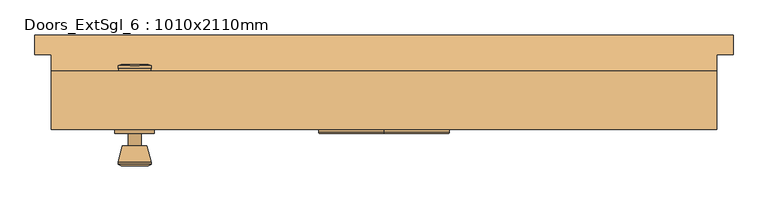
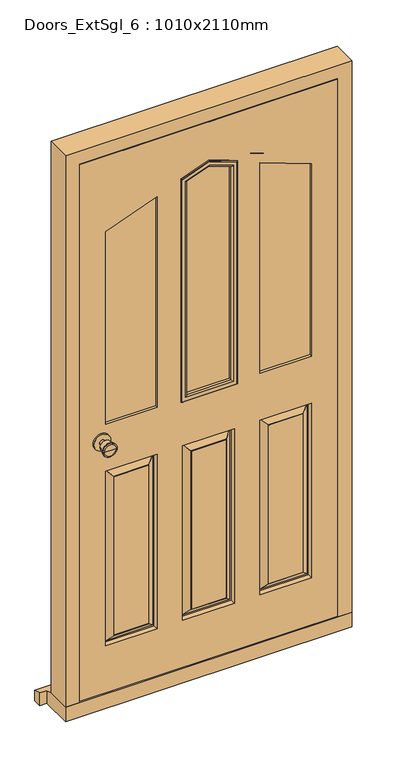
"""IFC4 building model written with IfcOpenShell, lengths in millimetres: door geometry, Doors_ExtSgl_6 : 1010x2110mm."""

from ifc_helpers import new_model, si_unit, point, frame, frame_2d, origin, place, context, project, spatial, polyline, circle_curve, ellipse_curve, trimmed, segment, composite_curve, outline, extrude, faceted_brep, source, transform, mapped, element, save
from ifc_brep_helpers import plane_surface, cylinder_surface, revolved_surface, advanced_brep


def doors_extsgl_6_1010x2110mm_b93c615f(model_context):
    return source(origin(), model_context, "Body", "SolidModel", [
        advanced_brep(
        [(-378.4666667, -18.4, 1000.0), (-368.4666667, -18.4, 1000.0), (-388.4666667, -18.4, 1000.0), (-357.9907991, -67.4, 1000.0), (-378.4666667, -67.4, 1000.0), (-398.9425342, -67.4, 1000.0), (-353.4666667, -65.5721319, 1000.0), (-403.4666667, -65.5721319, 1000.0), (-353.4666667, -62.1084537, 1000.0), (-403.4666667, -62.1084537, 1000.0), (-359.8304306, -37.4, 1000.0), (-397.1029027, -37.4, 1000.0), (-368.4666667, -37.4, 1000.0), (-388.4666667, -37.4, 1000.0)],
        [
            (0, 1),
            (1, 2, circle_curve(frame((-378.4666667, -18.4, 1000.0), z_axis=(0.0, 1.0, 0.0), x_axis=(-1.0, 0.0, 0.0)), 10.0)),
            (2, 0),
            (2, 1, circle_curve(frame((-378.4666667, -18.4, 1000.0), z_axis=(0.0, 1.0, 0.0), x_axis=(-1.0, 0.0, 0.0)), 10.0)),
            (3, 4),
            (4, 5),
            (5, 3, circle_curve(frame((-378.4666667, -67.4, 1000.0), z_axis=(0.0, -1.0, 0.0), x_axis=(-1.0, 0.0, 0.0)), 20.4758676)),
            (3, 5, circle_curve(frame((-378.4666667, -67.4, 1000.0), z_axis=(0.0, -1.0, 0.0), x_axis=(-1.0, 0.0, 0.0)), 20.4758676)),
            (6, 3),
            (5, 7),
            (7, 6, circle_curve(frame((-378.4666667, -65.5721319, 1000.0), z_axis=(0.0, -1.0, 0.0), x_axis=(-1.0, 0.0, 0.0)), 25.0)),
            (6, 7, circle_curve(frame((-378.4666667, -65.5721319, 1000.0), z_axis=(0.0, -1.0, 0.0), x_axis=(-1.0, 0.0, 0.0)), 25.0)),
            (8, 6),
            (7, 9),
            (9, 8, circle_curve(frame((-378.4666667, -62.1084537, 1000.0), z_axis=(0.0, -1.0, 0.0), x_axis=(-1.0, 0.0, 0.0)), 25.0)),
            (8, 9, circle_curve(frame((-378.4666667, -62.1084537, 1000.0), z_axis=(0.0, -1.0, 0.0), x_axis=(-1.0, 0.0, 0.0)), 25.0)),
            (10, 8),
            (9, 11),
            (11, 10, circle_curve(frame((-378.4666667, -37.4, 1000.0), z_axis=(0.0, -1.0, 0.0), x_axis=(-1.0, 0.0, 0.0)), 18.636236)),
            (10, 11, circle_curve(frame((-378.4666667, -37.4, 1000.0), z_axis=(0.0, -1.0, 0.0), x_axis=(-1.0, 0.0, 0.0)), 18.636236)),
            (12, 10),
            (11, 13),
            (13, 12, circle_curve(frame((-378.4666667, -37.4, 1000.0), z_axis=(0.0, -1.0, 0.0), x_axis=(-1.0, 0.0, 0.0)), 10.0)),
            (12, 13, circle_curve(frame((-378.4666667, -37.4, 1000.0), z_axis=(0.0, -1.0, 0.0), x_axis=(-1.0, 0.0, 0.0)), 10.0)),
            (1, 12),
            (13, 2),
        ],
        [
            plane_surface(frame((-378.4666667, -18.4, 1000.0), z_axis=(0.0, 1.0, 0.0), x_axis=(-1.0, 0.0, 0.0))),
            plane_surface(frame((-378.4666667, -67.4, 1000.0), z_axis=(0.0, -1.0, 0.0), x_axis=(-1.0, 0.0, 0.0))),
            revolved_surface(polyline([(-398.9425342, -67.4, 1000.0), (-403.4666667, -65.5721319, 1000.0)]), (-378.4666667, -18.4, 1000.0), (0.0, 1.0, 0.0)),
            cylinder_surface(frame((-378.4666667, -18.4, 1000.0), z_axis=(0.0, 1.0, 0.0), x_axis=(-1.0, 0.0, 0.0)), 25.0),
            revolved_surface(polyline([(-403.4666667, -62.1084537, 1000.0), (-397.1029027, -37.4, 1000.0)]), (-378.4666667, -18.4, 1000.0), (0.0, 1.0, 0.0)),
            plane_surface(frame((-378.4666667, -37.4, 1000.0), z_axis=(0.0, 1.0, 0.0), x_axis=(-1.0, 0.0, 0.0))),
            cylinder_surface(frame((-378.4666667, -18.4, 1000.0), z_axis=(0.0, 1.0, 0.0), x_axis=(-1.0, 0.0, 0.0)), 10.0),
        ],
        [
            (0, [[1, 2, 3]]),
            (0, [[-3, 4, -1]]),
            (1, [[5, 6, 7]]),
            (1, [[-6, -5, 8]]),
            (2, [[9, -7, 10, 11]]),
            (2, [[-10, -8, -9, 12]]),
            (3, [[13, -11, 14, 15]]),
            (3, [[-14, -12, -13, 16]]),
            (4, [[17, -15, 18, 19]]),
            (4, [[-18, -16, -17, 20]]),
            (5, [[21, -19, 22, 23]]),
            (5, [[-22, -20, -21, 24]]),
            (6, [[25, -23, 26, -2]]),
            (6, [[-26, -24, -25, -4]]),
        ],
    ),
        extrude(outline(composite_curve([segment(trimmed(circle_curve(frame_2d((1000.0, -378.4666667)), 30.0), [point((1000.0, -408.4666667))], [point((1000.0, -348.4666667))], False, "CARTESIAN"), True, "CONTINUOUS"), segment(trimmed(circle_curve(frame_2d((1000.0, -378.4666667)), 30.0), [point((1000.0, -348.4666667))], [point((1000.0, -408.4666667))], False, "CARTESIAN"), True, "CONTINUOUS")], self_intersect=False)), frame((0.0, -18.4, 0.0), z_axis=(0.0, 1.0, 0.0), x_axis=(0.0, 0.0, 1.0)), (0.0, 0.0, 1.0), 6.0),
        advanced_brep(
        [(-378.4666667, 37.6, 1000.0), (-388.4666667, 37.6, 1000.0), (-368.4666667, 37.6, 1000.0), (-357.9907991, 86.6, 1000.0), (-398.9425342, 86.6, 1000.0), (-378.4666667, 86.6, 1000.0), (-353.4666667, 84.7721319, 1000.0), (-403.4666667, 84.7721319, 1000.0), (-353.4666667, 81.3084537, 1000.0), (-403.4666667, 81.3084537, 1000.0), (-359.8304306, 56.6, 1000.0), (-397.1029027, 56.6, 1000.0), (-368.4666667, 56.6, 1000.0), (-388.4666667, 56.6, 1000.0)],
        [
            (0, 1),
            (1, 2, circle_curve(frame((-378.4666667, 37.6, 1000.0), z_axis=(0.0, -1.0, 0.0), x_axis=(-1.0, 0.0, 0.0)), 10.0)),
            (2, 0),
            (2, 1, circle_curve(frame((-378.4666667, 37.6, 1000.0), z_axis=(0.0, -1.0, 0.0), x_axis=(-1.0, 0.0, 0.0)), 10.0)),
            (3, 4, circle_curve(frame((-378.4666667, 86.6, 1000.0), z_axis=(0.0, 1.0, 0.0), x_axis=(-1.0, 0.0, 0.0)), 20.4758676)),
            (4, 5),
            (5, 3),
            (4, 3, circle_curve(frame((-378.4666667, 86.6, 1000.0), z_axis=(0.0, 1.0, 0.0), x_axis=(-1.0, 0.0, 0.0)), 20.4758676)),
            (6, 7, circle_curve(frame((-378.4666667, 84.7721319, 1000.0), z_axis=(0.0, 1.0, 0.0), x_axis=(-1.0, 0.0, 0.0)), 25.0)),
            (7, 4),
            (3, 6),
            (7, 6, circle_curve(frame((-378.4666667, 84.7721319, 1000.0), z_axis=(0.0, 1.0, 0.0), x_axis=(-1.0, 0.0, 0.0)), 25.0)),
            (8, 9, circle_curve(frame((-378.4666667, 81.3084537, 1000.0), z_axis=(0.0, 1.0, 0.0), x_axis=(-1.0, 0.0, 0.0)), 25.0)),
            (9, 7),
            (6, 8),
            (9, 8, circle_curve(frame((-378.4666667, 81.3084537, 1000.0), z_axis=(0.0, 1.0, 0.0), x_axis=(-1.0, 0.0, 0.0)), 25.0)),
            (10, 11, circle_curve(frame((-378.4666667, 56.6, 1000.0), z_axis=(0.0, 1.0, 0.0), x_axis=(-1.0, 0.0, 0.0)), 18.636236)),
            (11, 9),
            (8, 10),
            (11, 10, circle_curve(frame((-378.4666667, 56.6, 1000.0), z_axis=(0.0, 1.0, 0.0), x_axis=(-1.0, 0.0, 0.0)), 18.636236)),
            (12, 13, circle_curve(frame((-378.4666667, 56.6, 1000.0), z_axis=(0.0, 1.0, 0.0), x_axis=(-1.0, 0.0, 0.0)), 10.0)),
            (13, 11),
            (10, 12),
            (13, 12, circle_curve(frame((-378.4666667, 56.6, 1000.0), z_axis=(0.0, 1.0, 0.0), x_axis=(-1.0, 0.0, 0.0)), 10.0)),
            (1, 13),
            (12, 2),
        ],
        [
            plane_surface(frame((-378.4666667, 37.6, 1000.0), z_axis=(0.0, -1.0, 0.0), x_axis=(-1.0, 0.0, 0.0))),
            plane_surface(frame((-378.4666667, 86.6, 1000.0), z_axis=(0.0, 1.0, 0.0), x_axis=(-1.0, 0.0, 0.0))),
            revolved_surface(polyline([(-398.9425342, 86.6, 1000.0), (-403.4666667, 84.7721319, 1000.0)]), (-378.4666667, 37.6, 1000.0), (0.0, -1.0, 0.0)),
            cylinder_surface(frame((-378.4666667, 37.6, 1000.0), z_axis=(0.0, -1.0, 0.0), x_axis=(-1.0, 0.0, 0.0)), 25.0),
            revolved_surface(polyline([(-403.4666667, 81.3084537, 1000.0), (-397.1029027, 56.6, 1000.0)]), (-378.4666667, 37.6, 1000.0), (0.0, -1.0, 0.0)),
            plane_surface(frame((-378.4666667, 56.6, 1000.0), z_axis=(0.0, -1.0, 0.0), x_axis=(-1.0, 0.0, 0.0))),
            cylinder_surface(frame((-378.4666667, 37.6, 1000.0), z_axis=(0.0, -1.0, 0.0), x_axis=(-1.0, 0.0, 0.0)), 10.0),
        ],
        [
            (0, [[1, 2, 3]]),
            (0, [[-3, 4, -1]]),
            (1, [[5, 6, 7]]),
            (1, [[8, -7, -6]]),
            (2, [[9, 10, -5, 11]]),
            (2, [[12, -11, -8, -10]]),
            (3, [[13, 14, -9, 15]]),
            (3, [[16, -15, -12, -14]]),
            (4, [[17, 18, -13, 19]]),
            (4, [[20, -19, -16, -18]]),
            (5, [[21, 22, -17, 23]]),
            (5, [[24, -23, -20, -22]]),
            (6, [[-2, 25, -21, 26]]),
            (6, [[-4, -26, -24, -25]]),
        ],
    ),
        extrude(outline(composite_curve([segment(trimmed(circle_curve(frame_2d((1000.0, -378.4666667)), 30.0), [point((1000.0, -408.4666667))], [point((1000.0, -348.4666667))], False, "CARTESIAN"), True, "CONTINUOUS"), segment(trimmed(circle_curve(frame_2d((1000.0, -378.4666667)), 30.0), [point((1000.0, -348.4666667))], [point((1000.0, -408.4666667))], False, "CARTESIAN"), True, "CONTINUOUS")], self_intersect=False)), frame((0.0, 31.6, 0.0), z_axis=(0.0, 1.0, 0.0), x_axis=(0.0, 0.0, 1.0)), (0.0, 0.0, 1.0), 6.0),
        faceted_brep([(434.5333333, 76.6, 54.5), (505.0333333, 76.6, 54.5), (505.0333333, -12.4, 54.5), (456.5333333, -12.4, 54.5), (456.5333333, 34.6, 54.5), (434.5333333, 34.6, 54.5), (434.5333333, 76.6, 2039.5), (-434.4666667, 76.6, 2039.5), (-434.4666667, 76.6, 54.5), (-504.9666667, 76.6, 54.5), (-504.9666667, 76.6, 2110.0), (505.0333333, 76.6, 2110.0), (505.0333333, -12.4, 2110.0), (-504.9666667, -12.4, 2110.0), (-504.9666667, -12.4, 54.5), (-456.4666667, -12.4, 54.5), (-456.4666667, -12.4, 2061.5), (456.5333333, -12.4, 2061.5), (456.5333333, 34.6, 2061.5), (-456.4666667, 34.6, 2061.5), (-456.4666667, 34.6, 54.5), (-434.4666667, 34.6, 54.5), (-434.4666667, 34.6, 2039.5), (434.5333333, 34.6, 2039.5)], [[[0, 1, 2, 3, 4, 5]], [[1, 0, 6, 7, 8, 9, 10, 11]], [[2, 1, 11, 12]], [[3, 2, 12, 13, 14, 15, 16, 17]], [[4, 3, 17, 18]], [[5, 4, 18, 19, 20, 21, 22, 23]], [[0, 5, 23, 6]], [[8, 7, 22, 21]], [[9, 8, 21, 20, 15, 14]], [[10, 9, 14, 13]], [[16, 15, 20, 19]], [[11, 10, 13, 12]], [[17, 16, 19, 18]], [[7, 6, 23, 22]]]),
        faceted_brep([(453.5333333, -12.4, 58.5), (453.5333333, -12.4, 2058.5), (-454.3916961, -12.4, 2058.5), (-454.3916961, -12.4, 58.5), (-91.1333333, -12.4, 1058.5), (-91.1333333, -12.4, 1875.318047), (0.0333333, -12.4, 1908.5), (91.2, -12.4, 1875.318047), (91.2, -12.4, 1058.5), (363.5333333, -12.4, 1058.5), (181.2, -12.4, 1058.5), (181.2, -12.4, 1842.5607259), (363.5333333, -12.4, 1776.1968198), (-181.1333333, -12.4, 1842.5607259), (-181.1333333, -12.4, 1058.5), (-363.4666667, -12.4, 1058.5), (-363.4666667, -12.4, 1776.1968198), (-181.1333333, -12.4, 883.5), (-181.1333333, -12.4, 233.5), (-363.4666667, -12.4, 233.5), (-363.4666667, -12.4, 883.5), (363.5333333, -12.4, 883.5), (363.5333333, -12.4, 233.5), (181.2, -12.4, 233.5), (181.2, -12.4, 883.5), (91.2, -12.4, 883.5), (91.2, -12.4, 233.5), (-91.1333333, -12.4, 233.5), (-91.1333333, -12.4, 883.5), (-211.1333333, -12.4, 263.5), (-211.1333333, -12.4, 853.5), (-333.4666667, -12.4, 853.5), (-333.4666667, -12.4, 263.5), (333.5333333, -12.4, 263.5), (333.5333333, -12.4, 853.5), (211.2, -12.4, 853.5), (211.2, -12.4, 263.5), (61.2, -12.4, 263.5), (61.2, -12.4, 853.5), (-61.1333333, -12.4, 853.5), (-61.1333333, -12.4, 263.5), (453.5333333, 31.6, 58.5), (-454.3916961, 31.6, 58.5), (-454.3916961, 31.6, 2058.5), (453.5333333, 31.6, 2058.5), (-91.1333333, 31.6, 1058.5), (91.2, 31.6, 1058.5), (91.2, 31.6, 1875.318047), (0.0333333, 31.6, 1908.5), (-91.1333333, 31.6, 1875.318047), (363.5333333, 31.6, 1058.5), (363.5333333, 31.6, 1776.1968198), (181.2, 31.6, 1842.5607259), (181.2, 31.6, 1058.5), (-181.1333333, 31.6, 1842.5607259), (-363.4666667, 31.6, 1776.1968198), (-363.4666667, 31.6, 1058.5), (-181.1333333, 31.6, 1058.5), (181.2, 31.6, 883.5), (181.2, 31.6, 233.5), (363.5333333, 31.6, 233.5), (363.5333333, 31.6, 883.5), (-363.4666667, 31.6, 883.5), (-363.4666667, 31.6, 233.5), (-181.1333333, 31.6, 233.5), (-181.1333333, 31.6, 883.5), (-91.1333333, 31.6, 883.5), (-91.1333333, 31.6, 233.5), (91.2, 31.6, 233.5), (91.2, 31.6, 883.5), (211.2, 31.6, 263.5), (211.2, 31.6, 853.5), (333.5333333, 31.6, 853.5), (333.5333333, 31.6, 263.5), (-333.4666667, 31.6, 263.5), (-333.4666667, 31.6, 853.5), (-211.1333333, 31.6, 853.5), (-211.1333333, 31.6, 263.5), (-61.1333333, 31.6, 263.5), (-61.1333333, 31.6, 853.5), (61.2, 31.6, 853.5), (61.2, 31.6, 263.5), (184.2, 16.6, 880.5), (184.2, 16.6, 236.5), (209.2, 30.6, 855.5), (209.2, 30.6, 261.5), (189.2, 16.6, 241.5), (189.2, 16.6, 875.5), (211.2, 30.6, 263.5), (211.2, 30.6, 853.5), (360.5333333, 16.6, 236.5), (335.5333333, 30.6, 261.5), (355.5333333, 16.6, 241.5), (333.5333333, 30.6, 263.5), (360.5333333, 16.6, 880.5), (335.5333333, 30.6, 855.5), (355.5333333, 16.6, 875.5), (333.5333333, 30.6, 853.5), (-360.4666667, 16.6, 880.5), (-360.4666667, 16.6, 236.5), (-335.4666667, 30.6, 855.5), (-335.4666667, 30.6, 261.5), (-355.4666667, 16.6, 241.5), (-355.4666667, 16.6, 875.5), (-333.4666667, 30.6, 263.5), (-333.4666667, 30.6, 853.5), (-184.1333333, 16.6, 236.5), (-209.1333333, 30.6, 261.5), (-189.1333333, 16.6, 241.5), (-211.1333333, 30.6, 263.5), (-184.1333333, 16.6, 880.5), (-209.1333333, 30.6, 855.5), (-189.1333333, 16.6, 875.5), (-211.1333333, 30.6, 853.5), (-211.1333333, -11.4, 263.5), (-211.1333333, -11.4, 853.5), (-189.1333333, 2.6, 241.5), (-189.1333333, 2.6, 875.5), (-209.1333333, -11.4, 855.5), (-209.1333333, -11.4, 261.5), (-184.1333333, 2.6, 880.5), (-184.1333333, 2.6, 236.5), (-333.4666667, -11.4, 853.5), (-355.4666667, 2.6, 875.5), (-335.4666667, -11.4, 855.5), (-360.4666667, 2.6, 880.5), (-333.4666667, -11.4, 263.5), (-355.4666667, 2.6, 241.5), (-335.4666667, -11.4, 261.5), (-360.4666667, 2.6, 236.5), (360.5333333, 2.6, 880.5), (360.5333333, 2.6, 236.5), (335.5333333, -11.4, 855.5), (335.5333333, -11.4, 261.5), (355.5333333, 2.6, 241.5), (355.5333333, 2.6, 875.5), (333.5333333, -11.4, 263.5), (333.5333333, -11.4, 853.5), (184.2, 2.6, 236.5), (209.2, -11.4, 261.5), (189.2, 2.6, 241.5), (211.2, -11.4, 263.5), (184.2, 2.6, 880.5), (209.2, -11.4, 855.5), (189.2, 2.6, 875.5), (211.2, -11.4, 853.5), (-61.1333333, 30.6, 263.5), (-61.1333333, 30.6, 853.5), (-83.1333333, 16.6, 241.5), (-83.1333333, 16.6, 875.5), (-63.1333333, 30.6, 855.5), (-63.1333333, 30.6, 261.5), (-88.1333333, 16.6, 880.5), (-88.1333333, 16.6, 236.5), (61.2, 30.6, 853.5), (83.2, 16.6, 875.5), (63.2, 30.6, 855.5), (88.2, 16.6, 880.5), (61.2, 30.6, 263.5), (83.2, 16.6, 241.5), (63.2, 30.6, 261.5), (88.2, 16.6, 236.5), (88.2, 2.6, 880.5), (88.2, 2.6, 236.5), (63.2, -11.4, 855.5), (63.2, -11.4, 261.5), (83.2, 2.6, 241.5), (83.2, 2.6, 875.5), (61.2, -11.4, 263.5), (61.2, -11.4, 853.5), (-88.1333333, 2.6, 236.5), (-63.1333333, -11.4, 261.5), (-83.1333333, 2.6, 241.5), (-61.1333333, -11.4, 263.5), (-88.1333333, 2.6, 880.5), (-63.1333333, -11.4, 855.5), (-83.1333333, 2.6, 875.5), (-61.1333333, -11.4, 853.5)], [[[0, 1, 2, 3], [4, 5, 6, 7, 8], [9, 10, 11, 12], [13, 14, 15, 16], [17, 18, 19, 20], [21, 22, 23, 24], [25, 26, 27, 28]], [[29, 30, 31, 32]], [[33, 34, 35, 36]], [[37, 38, 39, 40]], [[41, 42, 43, 44], [45, 46, 47, 48, 49], [50, 51, 52, 53], [54, 55, 56, 57], [58, 59, 60, 61], [62, 63, 64, 65], [66, 67, 68, 69]], [[70, 71, 72, 73]], [[74, 75, 76, 77]], [[78, 79, 80, 81]], [[1, 0, 41, 44]], [[2, 1, 44, 43]], [[3, 2, 43, 42]], [[0, 3, 42, 41]], [[5, 4, 45, 49]], [[6, 5, 49, 48]], [[7, 6, 48, 47]], [[8, 7, 47, 46]], [[4, 8, 46, 45]], [[10, 9, 50, 53]], [[11, 10, 53, 52]], [[12, 11, 52, 51]], [[9, 12, 51, 50]], [[14, 13, 54, 57]], [[15, 14, 57, 56]], [[16, 15, 56, 55]], [[13, 16, 55, 54]], [[82, 83, 59, 58]], [[84, 85, 86, 87]], [[70, 88, 89, 71]], [[59, 83, 90, 60]], [[86, 85, 91, 92]], [[88, 70, 73, 93]], [[60, 90, 94, 61]], [[92, 91, 95, 96]], [[93, 73, 72, 97]], [[82, 58, 61, 94]], [[83, 82, 94, 90], [87, 86, 92, 96]], [[84, 87, 96, 95]], [[85, 84, 95, 91], [89, 88, 93, 97]], [[71, 89, 97, 72]], [[98, 99, 63, 62]], [[100, 101, 102, 103]], [[74, 104, 105, 75]], [[63, 99, 106, 64]], [[102, 101, 107, 108]], [[104, 74, 77, 109]], [[64, 106, 110, 65]], [[108, 107, 111, 112]], [[109, 77, 76, 113]], [[98, 62, 65, 110]], [[99, 98, 110, 106], [103, 102, 108, 112]], [[100, 103, 112, 111]], [[101, 100, 111, 107], [105, 104, 109, 113]], [[75, 105, 113, 76]], [[114, 115, 30, 29]], [[116, 117, 118, 119]], [[17, 120, 121, 18]], [[30, 115, 122, 31]], [[118, 117, 123, 124]], [[120, 17, 20, 125]], [[31, 122, 126, 32]], [[124, 123, 127, 128]], [[125, 20, 19, 129]], [[114, 29, 32, 126]], [[119, 118, 124, 128], [115, 114, 126, 122]], [[116, 119, 128, 127]], [[121, 120, 125, 129], [117, 116, 127, 123]], [[18, 121, 129, 19]], [[130, 131, 22, 21]], [[132, 133, 134, 135]], [[33, 136, 137, 34]], [[22, 131, 138, 23]], [[134, 133, 139, 140]], [[136, 33, 36, 141]], [[23, 138, 142, 24]], [[140, 139, 143, 144]], [[141, 36, 35, 145]], [[130, 21, 24, 142]], [[131, 130, 142, 138], [135, 134, 140, 144]], [[132, 135, 144, 143]], [[133, 132, 143, 139], [137, 136, 141, 145]], [[34, 137, 145, 35]], [[146, 147, 79, 78]], [[148, 149, 150, 151]], [[66, 152, 153, 67]], [[79, 147, 154, 80]], [[150, 149, 155, 156]], [[152, 66, 69, 157]], [[80, 154, 158, 81]], [[156, 155, 159, 160]], [[157, 69, 68, 161]], [[146, 78, 81, 158]], [[151, 150, 156, 160], [147, 146, 158, 154]], [[148, 151, 160, 159]], [[153, 152, 157, 161], [149, 148, 159, 155]], [[67, 153, 161, 68]], [[162, 163, 26, 25]], [[164, 165, 166, 167]], [[37, 168, 169, 38]], [[26, 163, 170, 27]], [[166, 165, 171, 172]], [[168, 37, 40, 173]], [[27, 170, 174, 28]], [[172, 171, 175, 176]], [[173, 40, 39, 177]], [[162, 25, 28, 174]], [[163, 162, 174, 170], [167, 166, 172, 176]], [[164, 167, 176, 175]], [[165, 164, 175, 171], [169, 168, 173, 177]], [[38, 169, 177, 39]]]),
        faceted_brep([(530.0333333, 131.6, 0.0), (530.0333333, 131.6, 38.5947221), (530.0333333, 101.6, 47.2703282), (530.0333333, 101.6, 0.0), (-529.9666667, 131.6, 38.5947221), (-529.9666667, 131.6, 0.0), (-529.9666667, 101.6, 0.0), (-529.9666667, 101.6, 47.2703282), (505.0333333, 101.6, 0.0), (505.0333333, -12.4, 0.0), (-504.9666667, -12.4, 0.0), (-504.9666667, 101.6, 0.0), (-504.9666667, 101.6, 47.2703282), (-504.9666667, 76.6, 54.5), (505.0333333, 76.6, 54.5), (505.0333333, 101.6, 47.2703282), (-504.9666667, -12.4, 54.5), (505.0333333, -12.4, 54.5)], [[[0, 1, 2, 3]], [[4, 5, 6, 7]], [[5, 0, 3, 8, 9, 10, 11, 6]], [[1, 0, 5, 4]], [[1, 4, 7, 12, 13, 14, 15, 2]], [[13, 16, 17, 14]], [[16, 10, 9, 17]], [[12, 11, 10, 16, 13]], [[11, 12, 7, 6]], [[8, 15, 14, 17, 9]], [[15, 8, 3, 2]]]),
        extrude(outline(polyline([(1058.5, -91.1333333), (1058.5, 91.2), (1875.318047, 91.2), (1908.5, 0.0333333), (1875.318047, -91.1333333), (1058.5, -91.1333333)])), frame((0.0, -2.4, 0.0), z_axis=(0.0, 1.0, 0.0), x_axis=(0.0, 0.0, 1.0)), (0.0, 0.0, 1.0), 24.0),
        extrude(outline(polyline([(1776.1968198, 363.5333333), (1842.5607259, 181.2), (1058.5, 181.2), (1058.5, 363.5333333), (1776.1968198, 363.5333333)])), frame((0.0, -2.4, 0.0), z_axis=(0.0, 1.0, 0.0), x_axis=(0.0, 0.0, 1.0)), (0.0, 0.0, 1.0), 24.0),
        extrude(outline(polyline([(1058.5, -181.1333333), (1842.5607259, -181.1333333), (1776.1968198, -363.4666667), (1058.5, -363.4666667), (1058.5, -181.1333333)])), frame((0.0, -2.4, 0.0), z_axis=(0.0, 1.0, 0.0), x_axis=(0.0, 0.0, 1.0)), (0.0, 0.0, 1.0), 24.0),
        advanced_brep(
        [(-99.1333333, 35.6, 1050.5), (-99.1333333, 31.6, 1050.5), (-99.1333333, 31.6, 1880.9197073), (-99.1333333, 35.6, 1880.9197073), (-97.1333333, 37.6, 1052.5), (-97.1333333, 37.6, 1879.5192922), (-79.1333333, 32.6, 1070.5), (-84.1333333, 37.6, 1065.5), (-84.1333333, 37.6, 1870.4165942), (-79.1333333, 32.6, 1866.9155565), (-79.1333333, 21.6, 1070.5), (-79.1333333, 21.6, 1866.9155565), (-91.1333333, 31.6, 1058.5), (-91.1333333, 21.6, 1058.5), (-91.1333333, 21.6, 1875.318047), (-91.1333333, 31.6, 1875.318047), (0.0333333, 31.6, 1917.0134222), (0.0333333, 35.6, 1917.0134222), (0.0333333, 37.6, 1914.8850666), (0.0333333, 37.6, 1901.0507556), (0.0333333, 32.6, 1895.7298667), (0.0333333, 21.6, 1895.7298667), (0.0333333, 21.6, 1908.5), (0.0333333, 31.6, 1908.5), (99.2, 31.6, 1880.9197073), (99.2, 35.6, 1880.9197073), (97.2, 37.6, 1879.5192922), (97.2, 37.6, 1052.5), (84.2, 37.6, 1870.4165942), (84.2, 37.6, 1065.5), (79.2, 32.6, 1866.9155565), (79.2, 21.6, 1866.9155565), (91.2, 21.6, 1875.318047), (91.2, 21.6, 1058.5), (79.2, 21.6, 1070.5), (91.2, 31.6, 1875.318047), (99.2, 31.6, 1050.5), (91.2, 31.6, 1058.5), (99.2, 35.6, 1050.5), (79.2, 32.6, 1070.5)],
        [
            (0, 1),
            (1, 2),
            (2, 3),
            (3, 0),
            (4, 0, ellipse_curve(frame((-97.1333333, 35.6, 1052.5), z_axis=(-0.7071067811865476, 0.0, 0.7071067811865474), x_axis=(-0.7071067811865471, 0.0, -0.7071067811865478)), 2.8284271, 2.0)),
            (3, 5, ellipse_curve(frame((-97.1333333, 35.6, 1879.5192922), z_axis=(-0.5735764363510456, 0.0, -0.8191520442889918), x_axis=(0.8191520442889916, 0.0, -0.5735764363510464)), 2.4415492, 2.0)),
            (5, 4),
            (6, 7, ellipse_curve(frame((-84.1333333, 32.6, 1065.5), z_axis=(-0.7071067811865476, 0.0, 0.7071067811865474), x_axis=(-0.7071067811865471, 0.0, -0.7071067811865478)), 7.0710678, 5.0)),
            (7, 8),
            (8, 9, ellipse_curve(frame((-84.1333333, 32.6, 1870.4165942), z_axis=(-0.5735764363510456, 0.0, -0.8191520442889918), x_axis=(0.8191520442889916, 0.0, -0.5735764363510464)), 6.1038729, 5.0)),
            (9, 6),
            (10, 6),
            (9, 11),
            (11, 10),
            (12, 13),
            (13, 14),
            (14, 15),
            (15, 12),
            (2, 16),
            (16, 17),
            (17, 3),
            (17, 18, ellipse_curve(frame((0.0333333, 35.6, 1914.8850666), z_axis=(-1.0, 0.0, 0.0), x_axis=(0.0, 0.0, -0.9999999999999999)), 2.1283555, 2.0)),
            (18, 5),
            (8, 19),
            (19, 20, ellipse_curve(frame((0.0333333, 32.6, 1901.0507556), z_axis=(-1.0, 0.0, 0.0), x_axis=(0.0, 0.0, -0.9999999999999999)), 5.3208889, 5.0)),
            (20, 9),
            (20, 21),
            (21, 11),
            (14, 22),
            (22, 23),
            (23, 15),
            (16, 24),
            (24, 25),
            (25, 17),
            (25, 26, ellipse_curve(frame((97.2, 35.6, 1879.5192922), z_axis=(-0.5735764363510465, 0.0, 0.8191520442889915), x_axis=(-0.8191520442889916, 0.0, -0.5735764363510464)), 2.4415492, 2.0)),
            (26, 18),
            (26, 27),
            (27, 4),
            (28, 19),
            (7, 29),
            (29, 28),
            (28, 30, ellipse_curve(frame((84.2, 32.6, 1870.4165942), z_axis=(-0.5735764363510465, 0.0, 0.8191520442889915), x_axis=(-0.8191520442889916, 0.0, -0.5735764363510464)), 6.1038729, 5.0)),
            (30, 20),
            (30, 31),
            (31, 21),
            (32, 22),
            (13, 33),
            (33, 32),
            (31, 34),
            (34, 10),
            (32, 35),
            (35, 23),
            (1, 36),
            (36, 24),
            (35, 37),
            (37, 12),
            (36, 38),
            (38, 25),
            (38, 27, ellipse_curve(frame((97.2, 35.6, 1052.5), z_axis=(0.7071067811865474, 0.0, 0.7071067811865476), x_axis=(-0.7071067811865475, 0.0, 0.7071067811865475)), 2.8284271, 2.0)),
            (29, 39, ellipse_curve(frame((84.2, 32.6, 1065.5), z_axis=(0.7071067811865474, 0.0, 0.7071067811865476), x_axis=(-0.7071067811865475, 0.0, 0.7071067811865475)), 7.0710678, 5.0)),
            (39, 30),
            (39, 34),
            (33, 37),
            (0, 38),
            (6, 39),
        ],
        [
            plane_surface(frame((-99.1333333, 31.6, 1050.5), z_axis=(-1.0, 0.0, 0.0), x_axis=(0.0, 0.0, 1.0))),
            cylinder_surface(frame((-97.1333333, 35.6, 1058.5), z_axis=(0.0, 0.0, -1.0), x_axis=(-1.0, 0.0, 0.0)), 2.0),
            cylinder_surface(frame((-84.1333333, 32.6, 1058.5), z_axis=(0.0, 0.0, -1.0), x_axis=(-1.0, 0.0, 0.0)), 5.0),
            plane_surface(frame((-79.1333333, 32.6, 1070.5), z_axis=(1.0, 0.0, 0.0), x_axis=(0.0, 0.0, 1.0))),
            plane_surface(frame((-91.1333333, 21.6, 1058.5), z_axis=(-1.0, 0.0, 0.0), x_axis=(0.0, 0.0, 1.0))),
            plane_surface(frame((-99.1333333, 31.6, 1880.9197073), z_axis=(-0.3420201433256681, 0.0, 0.9396926207859086), x_axis=(0.9396926207859086, 0.0, 0.3420201433256681))),
            cylinder_surface(frame((-93.1854542, 35.6, 1880.9562027), z_axis=(-0.9396926207859082, 0.0, -0.3420201433256694), x_axis=(-0.3420201433256694, 0.0, 0.9396926207859082)), 2.0),
            cylinder_surface(frame((-88.7391923, 32.6, 1868.7401986), z_axis=(-0.9396926207859082, 0.0, -0.3420201433256694), x_axis=(-0.3420201433256694, 0.0, 0.9396926207859082)), 5.0),
            plane_surface(frame((-79.1333333, 32.6, 1866.9155565), z_axis=(0.34202014332567027, 0.0, -0.939692620785908), x_axis=(0.939692620785908, 0.0, 0.34202014332567027))),
            plane_surface(frame((-91.1333333, 21.6, 1875.318047), z_axis=(-0.34202014332566794, 0.0, 0.9396926207859088), x_axis=(0.9396926207859088, 0.0, 0.34202014332566794))),
            plane_surface(frame((0.0333333, 31.6, 1917.0134222), z_axis=(0.34202014332567027, 0.0, 0.9396926207859079), x_axis=(0.9396926207859079, 0.0, -0.34202014332567027))),
            cylinder_surface(frame((2.0854542, 35.6, 1914.1381557), z_axis=(-0.9396926207859086, 0.0, 0.3420201433256681), x_axis=(0.3420201433256681, 0.0, 0.9396926207859086)), 2.0),
            plane_surface(frame((0.0333333, 37.6, 1914.8850666), z_axis=(0.0, 1.0, 0.0), x_axis=(0.9396926207859083, 0.0, -0.3420201433256691))),
            cylinder_surface(frame((-2.3608077, 32.6, 1901.9221517), z_axis=(-0.9396926207859086, 0.0, 0.3420201433256681), x_axis=(0.3420201433256681, 0.0, 0.9396926207859086)), 5.0),
            plane_surface(frame((0.0333333, 32.6, 1895.7298667), z_axis=(-0.3420201433256694, 0.0, -0.9396926207859082), x_axis=(0.9396926207859082, 0.0, -0.3420201433256694))),
            plane_surface(frame((0.0333333, 21.6, 1895.7298667), z_axis=(0.0, -1.0, 0.0), x_axis=(0.9396926207859081, 0.0, -0.34202014332566955))),
            plane_surface(frame((0.0333333, 21.6, 1908.5), z_axis=(0.3420201433256692, 0.0, 0.9396926207859083), x_axis=(0.9396926207859083, 0.0, -0.3420201433256692))),
            plane_surface(frame((0.0333333, 31.6, 1908.5), z_axis=(0.0, -1.0000000000000002, 0.0), x_axis=(0.9396926207859083, 0.0, -0.3420201433256692))),
            plane_surface(frame((99.2, 31.6, 1880.9197073), z_axis=(1.0, 0.0, 0.0), x_axis=(0.0, 0.0, -1.0))),
            cylinder_surface(frame((97.2, 35.6, 1875.318047), z_axis=(0.0, 0.0, 1.0), x_axis=(1.0, 0.0, 0.0)), 2.0),
            cylinder_surface(frame((84.2, 32.6, 1875.318047), z_axis=(0.0, 0.0, 1.0), x_axis=(1.0, 0.0, 0.0)), 5.0),
            plane_surface(frame((79.2, 32.6, 1866.9155565), z_axis=(-1.0, 0.0, 0.0), x_axis=(0.0, 0.0, -1.0))),
            plane_surface(frame((91.2, 21.6, 1875.318047), z_axis=(1.0, 0.0, 0.0), x_axis=(0.0, 0.0, -1.0))),
            plane_surface(frame((99.2, 31.6, 1050.5), z_axis=(0.0, 0.0, -1.0), x_axis=(-1.0, 0.0, 0.0))),
            cylinder_surface(frame((91.2, 35.6, 1052.5), z_axis=(1.0, 0.0, 0.0), x_axis=(0.0, 0.0, -1.0)), 2.0),
            cylinder_surface(frame((91.2, 32.6, 1065.5), z_axis=(1.0, 0.0, 0.0), x_axis=(0.0, 0.0, -1.0)), 5.0),
            plane_surface(frame((79.2, 32.6, 1070.5), z_axis=(0.0, 0.0, 1.0), x_axis=(-1.0, 0.0, 0.0))),
            plane_surface(frame((91.2, 21.6, 1058.5), z_axis=(0.0, 0.0, -1.0), x_axis=(-1.0, 0.0, 0.0))),
        ],
        [
            (0, [[1, 2, 3, 4]]),
            (1, [[5, -4, 6, 7]]),
            (2, [[8, 9, 10, 11]]),
            (3, [[12, -11, 13, 14]]),
            (4, [[15, 16, 17, 18]]),
            (5, [[-3, 19, 20, 21]]),
            (6, [[-6, -21, 22, 23]]),
            (7, [[-10, 24, 25, 26]]),
            (8, [[-13, -26, 27, 28]]),
            (9, [[-17, 29, 30, 31]]),
            (10, [[-20, 32, 33, 34]]),
            (11, [[-22, -34, 35, 36]]),
            (12, [[-7, -23, -36, 37, 38], [39, -24, -9, 40, 41]]),
            (13, [[-25, -39, 42, 43]]),
            (14, [[-27, -43, 44, 45]]),
            (15, [[46, -29, -16, 47, 48], [-14, -28, -45, 49, 50]]),
            (16, [[-30, -46, 51, 52]]),
            (17, [[-32, -19, -2, 53, 54], [-18, -31, -52, 55, 56]]),
            (18, [[-33, -54, 57, 58]]),
            (19, [[-35, -58, 59, -37]]),
            (20, [[-42, -41, 60, 61]]),
            (21, [[-44, -61, 62, -49]]),
            (22, [[-51, -48, 63, -55]]),
            (23, [[-57, -53, -1, 64]]),
            (24, [[-59, -64, -5, -38]]),
            (25, [[-60, -40, -8, 65]]),
            (26, [[-62, -65, -12, -50]]),
            (27, [[-63, -47, -15, -56]]),
        ],
    ),
        advanced_brep(
        [(99.2, -16.4, 1050.5), (99.2, -12.4, 1050.5), (99.2, -12.4, 1880.9197073), (99.2, -16.4, 1880.9197073), (97.2, -18.4, 1052.5), (97.2, -18.4, 1879.5192922), (79.2, -13.4, 1070.5), (84.2, -18.4, 1065.5), (84.2, -18.4, 1870.4165942), (79.2, -13.4, 1866.9155565), (79.2, -2.4, 1070.5), (79.2, -2.4, 1866.9155565), (91.2, -12.4, 1058.5), (91.2, -2.4, 1058.5), (91.2, -2.4, 1875.318047), (91.2, -12.4, 1875.318047), (0.0333333, -12.4, 1917.0134222), (0.0333333, -16.4, 1917.0134222), (0.0333333, -18.4, 1914.8850666), (0.0333333, -18.4, 1901.0507556), (0.0333333, -13.4, 1895.7298667), (0.0333333, -2.4, 1895.7298667), (0.0333333, -2.4, 1908.5), (0.0333333, -12.4, 1908.5), (-99.1333333, -12.4, 1880.9197073), (-99.1333333, -16.4, 1880.9197073), (-97.1333333, -18.4, 1879.5192922), (-97.1333333, -18.4, 1052.5), (-84.1333333, -18.4, 1870.4165942), (-84.1333333, -18.4, 1065.5), (-79.1333333, -13.4, 1866.9155565), (-79.1333333, -2.4, 1866.9155565), (-91.1333333, -2.4, 1875.318047), (-91.1333333, -2.4, 1058.5), (-79.1333333, -2.4, 1070.5), (-91.1333333, -12.4, 1875.318047), (-99.1333333, -12.4, 1050.5), (-91.1333333, -12.4, 1058.5), (-99.1333333, -16.4, 1050.5), (-79.1333333, -13.4, 1070.5)],
        [
            (0, 1),
            (1, 2),
            (2, 3),
            (3, 0),
            (4, 0, ellipse_curve(frame((97.2, -16.4, 1052.5), z_axis=(0.7071067811865472, 0.0, 0.7071067811865477), x_axis=(0.7071067811865476, 0.0, -0.7071067811865474)), 2.8284271, 2.0)),
            (3, 5, ellipse_curve(frame((97.2, -16.4, 1879.5192922), z_axis=(0.5735764363510465, 0.0, -0.8191520442889915), x_axis=(-0.8191520442889915, 0.0, -0.5735764363510466)), 2.4415492, 2.0)),
            (5, 4),
            (6, 7, ellipse_curve(frame((84.2, -13.4, 1065.5), z_axis=(0.7071067811865472, 0.0, 0.7071067811865477), x_axis=(0.7071067811865476, 0.0, -0.7071067811865474)), 7.0710678, 5.0)),
            (7, 8),
            (8, 9, ellipse_curve(frame((84.2, -13.4, 1870.4165942), z_axis=(0.5735764363510465, 0.0, -0.8191520442889915), x_axis=(-0.8191520442889915, 0.0, -0.5735764363510466)), 6.1038729, 5.0)),
            (9, 6),
            (10, 6),
            (9, 11),
            (11, 10),
            (12, 13),
            (13, 14),
            (14, 15),
            (15, 12),
            (2, 16),
            (16, 17),
            (17, 3),
            (17, 18, ellipse_curve(frame((0.0333333, -16.4, 1914.8850666), z_axis=(1.0, 0.0, 0.0), x_axis=(0.0, 0.0, -1.0)), 2.1283555, 2.0)),
            (18, 5),
            (8, 19),
            (19, 20, ellipse_curve(frame((0.0333333, -13.4, 1901.0507556), z_axis=(1.0, 0.0, 0.0), x_axis=(0.0, 0.0, -1.0)), 5.3208889, 5.0)),
            (20, 9),
            (20, 21),
            (21, 11),
            (14, 22),
            (22, 23),
            (23, 15),
            (16, 24),
            (24, 25),
            (25, 17),
            (25, 26, ellipse_curve(frame((-97.1333333, -16.4, 1879.5192922), z_axis=(0.573576436351046, 0.0, 0.8191520442889919), x_axis=(0.8191520442889917, 0.0, -0.5735764363510462)), 2.4415492, 2.0)),
            (26, 18),
            (26, 27),
            (27, 4),
            (28, 19),
            (7, 29),
            (29, 28),
            (28, 30, ellipse_curve(frame((-84.1333333, -13.4, 1870.4165942), z_axis=(0.573576436351046, 0.0, 0.8191520442889919), x_axis=(0.8191520442889917, 0.0, -0.5735764363510462)), 6.1038729, 5.0)),
            (30, 20),
            (30, 31),
            (31, 21),
            (32, 22),
            (13, 33),
            (33, 32),
            (31, 34),
            (34, 10),
            (32, 35),
            (35, 23),
            (1, 36),
            (36, 24),
            (35, 37),
            (37, 12),
            (36, 38),
            (38, 25),
            (38, 27, ellipse_curve(frame((-97.1333333, -16.4, 1052.5), z_axis=(-0.7071067811865477, 0.0, 0.7071067811865474), x_axis=(0.7071067811865472, 0.0, 0.7071067811865477)), 2.8284271, 2.0)),
            (29, 39, ellipse_curve(frame((-84.1333333, -13.4, 1065.5), z_axis=(-0.7071067811865477, 0.0, 0.7071067811865474), x_axis=(0.7071067811865472, 0.0, 0.7071067811865477)), 7.0710678, 5.0)),
            (39, 30),
            (39, 34),
            (33, 37),
            (0, 38),
            (6, 39),
        ],
        [
            plane_surface(frame((99.2, -12.4, 1050.5), z_axis=(1.0, 0.0, 0.0), x_axis=(0.0, 0.0, 1.0))),
            cylinder_surface(frame((97.2, -16.4, 1058.5), z_axis=(0.0, 0.0, -1.0), x_axis=(1.0, 0.0, 0.0)), 2.0),
            cylinder_surface(frame((84.2, -13.4, 1058.5), z_axis=(0.0, 0.0, -1.0), x_axis=(1.0, 0.0, 0.0)), 5.0),
            plane_surface(frame((79.2, -13.4, 1070.5), z_axis=(-1.0, 0.0, 0.0), x_axis=(0.0, 0.0, 1.0))),
            plane_surface(frame((91.2, -2.4, 1058.5), z_axis=(1.0, 0.0, 0.0), x_axis=(0.0, 0.0, 1.0))),
            plane_surface(frame((99.2, -12.4, 1880.9197073), z_axis=(0.34202014332566794, 0.0, 0.9396926207859088), x_axis=(-0.9396926207859088, 0.0, 0.34202014332566794))),
            cylinder_surface(frame((93.2521209, -16.4, 1880.9562027), z_axis=(0.9396926207859088, 0.0, -0.342020143325668), x_axis=(0.342020143325668, 0.0, 0.9396926207859088)), 2.0),
            cylinder_surface(frame((88.805859, -13.4, 1868.7401986), z_axis=(0.9396926207859088, 0.0, -0.342020143325668), x_axis=(0.342020143325668, 0.0, 0.9396926207859088)), 5.0),
            plane_surface(frame((79.2, -13.4, 1866.9155565), z_axis=(-0.34202014332566766, 0.0, -0.9396926207859088), x_axis=(-0.9396926207859088, 0.0, 0.34202014332566766))),
            plane_surface(frame((91.2, -2.4, 1875.318047), z_axis=(0.34202014332567027, 0.0, 0.9396926207859079), x_axis=(-0.9396926207859079, 0.0, 0.34202014332567027))),
            plane_surface(frame((0.0333333, -12.4, 1917.0134222), z_axis=(-0.34202014332566916, 0.0, 0.9396926207859082), x_axis=(-0.9396926207859082, 0.0, -0.34202014332566916))),
            cylinder_surface(frame((-2.0187875, -16.4, 1914.1381557), z_axis=(0.9396926207859085, 0.0, 0.3420201433256686), x_axis=(-0.3420201433256686, 0.0, 0.9396926207859085)), 2.0),
            plane_surface(frame((0.0333333, -18.4, 1914.8850666), z_axis=(0.0, -1.0000000000000002, 0.0), x_axis=(-0.939692620785909, 0.0, -0.34202014332566727))),
            cylinder_surface(frame((2.4274743, -13.4, 1901.9221517), z_axis=(0.9396926207859085, 0.0, 0.3420201433256686), x_axis=(-0.3420201433256686, 0.0, 0.9396926207859085)), 5.0),
            plane_surface(frame((0.0333333, -13.4, 1895.7298667), z_axis=(0.3420201433256686, 0.0, -0.9396926207859084), x_axis=(-0.9396926207859084, 0.0, -0.3420201433256686))),
            plane_surface(frame((0.0333333, -2.4, 1895.7298667), z_axis=(0.0, 1.0000000000000002, 0.0), x_axis=(-0.9396926207859086, 0.0, -0.34202014332566827))),
            plane_surface(frame((0.0333333, -2.4, 1908.5), z_axis=(-0.3420201433256662, 0.0, 0.9396926207859093), x_axis=(-0.9396926207859093, 0.0, -0.3420201433256662))),
            plane_surface(frame((0.0333333, -12.4, 1908.5), z_axis=(0.0, 1.0, 0.0), x_axis=(-0.9396926207859093, 0.0, -0.3420201433256662))),
            plane_surface(frame((-99.1333333, -12.4, 1880.9197073), z_axis=(-1.0, 0.0, 0.0), x_axis=(0.0, 0.0, -1.0))),
            cylinder_surface(frame((-97.1333333, -16.4, 1875.318047), z_axis=(0.0, 0.0, 1.0), x_axis=(-1.0, 0.0, 0.0)), 2.0),
            cylinder_surface(frame((-84.1333333, -13.4, 1875.318047), z_axis=(0.0, 0.0, 1.0), x_axis=(-1.0, 0.0, 0.0)), 5.0),
            plane_surface(frame((-79.1333333, -13.4, 1866.9155565), z_axis=(1.0, 0.0, 0.0), x_axis=(0.0, 0.0, -1.0))),
            plane_surface(frame((-91.1333333, -2.4, 1875.318047), z_axis=(-1.0, 0.0, 0.0), x_axis=(0.0, 0.0, -1.0))),
            plane_surface(frame((-99.1333333, -12.4, 1050.5), z_axis=(0.0, 0.0, -1.0), x_axis=(1.0, 0.0, 0.0))),
            cylinder_surface(frame((-91.1333333, -16.4, 1052.5), z_axis=(-1.0, 0.0, 0.0), x_axis=(0.0, 0.0, -1.0)), 2.0),
            cylinder_surface(frame((-91.1333333, -13.4, 1065.5), z_axis=(-1.0, 0.0, 0.0), x_axis=(0.0, 0.0, -1.0)), 5.0),
            plane_surface(frame((-79.1333333, -13.4, 1070.5), z_axis=(0.0, 0.0, 1.0), x_axis=(1.0, 0.0, 0.0))),
            plane_surface(frame((-91.1333333, -2.4, 1058.5), z_axis=(0.0, 0.0, -1.0), x_axis=(1.0, 0.0, 0.0))),
        ],
        [
            (0, [[1, 2, 3, 4]]),
            (1, [[5, -4, 6, 7]]),
            (2, [[8, 9, 10, 11]]),
            (3, [[12, -11, 13, 14]]),
            (4, [[15, 16, 17, 18]]),
            (5, [[-3, 19, 20, 21]]),
            (6, [[-6, -21, 22, 23]]),
            (7, [[-10, 24, 25, 26]]),
            (8, [[-13, -26, 27, 28]]),
            (9, [[-17, 29, 30, 31]]),
            (10, [[-20, 32, 33, 34]]),
            (11, [[-22, -34, 35, 36]]),
            (12, [[-7, -23, -36, 37, 38], [39, -24, -9, 40, 41]]),
            (13, [[-25, -39, 42, 43]]),
            (14, [[-27, -43, 44, 45]]),
            (15, [[46, -29, -16, 47, 48], [-14, -28, -45, 49, 50]]),
            (16, [[-30, -46, 51, 52]]),
            (17, [[-32, -19, -2, 53, 54], [-18, -31, -52, 55, 56]]),
            (18, [[-33, -54, 57, 58]]),
            (19, [[-35, -58, 59, -37]]),
            (20, [[-42, -41, 60, 61]]),
            (21, [[-44, -61, 62, -49]]),
            (22, [[-51, -48, 63, -55]]),
            (23, [[-57, -53, -1, 64]]),
            (24, [[-59, -64, -5, -38]]),
            (25, [[-60, -40, -8, 65]]),
            (26, [[-62, -65, -12, -50]]),
            (27, [[-63, -47, -15, -56]]),
        ],
    ),
        advanced_brep(
        [(371.5333333, 35.6, 1781.7984801), (371.5333333, 31.6, 1781.7984801), (371.5333333, 31.6, 1050.5), (371.5333333, 35.6, 1050.5), (369.5333333, 37.6, 1780.3980651), (369.5333333, 37.6, 1052.5), (351.5333333, 32.6, 1767.7943294), (356.5333333, 37.6, 1771.2953671), (356.5333333, 37.6, 1065.5), (351.5333333, 32.6, 1070.5), (351.5333333, 21.6, 1767.7943294), (351.5333333, 21.6, 1070.5), (363.5333333, 31.6, 1776.1968198), (363.5333333, 21.6, 1776.1968198), (363.5333333, 21.6, 1058.5), (363.5333333, 31.6, 1058.5), (173.2, 31.6, 1050.5), (173.2, 35.6, 1050.5), (175.2, 37.6, 1052.5), (188.2, 37.6, 1065.5), (193.2, 32.6, 1070.5), (193.2, 21.6, 1070.5), (181.2, 21.6, 1058.5), (181.2, 31.6, 1058.5), (173.2, 31.6, 1853.9859099), (173.2, 35.6, 1853.9859099), (175.2, 37.6, 1851.1296139), (188.2, 37.6, 1832.5636898), (193.2, 32.6, 1825.4229498), (193.2, 21.6, 1825.4229498), (181.2, 21.6, 1842.5607259), (181.2, 31.6, 1842.5607259)],
        [
            (0, 1),
            (1, 2),
            (2, 3),
            (3, 0),
            (4, 0, ellipse_curve(frame((369.5333333, 35.6, 1780.3980651), z_axis=(0.5735764363510453, 0.0, -0.8191520442889922), x_axis=(0.8191520442889922, 0.0, 0.5735764363510456)), 2.4415492, 2.0)),
            (3, 5, ellipse_curve(frame((369.5333333, 35.6, 1052.5), z_axis=(0.7071067811865475, 0.0, 0.7071067811865475), x_axis=(-0.7071067811865474, 0.0, 0.7071067811865476)), 2.8284271, 2.0)),
            (5, 4),
            (6, 7, ellipse_curve(frame((356.5333333, 32.6, 1771.2953671), z_axis=(0.5735764363510453, 0.0, -0.8191520442889922), x_axis=(0.8191520442889922, 0.0, 0.5735764363510456)), 6.1038729, 5.0)),
            (7, 8),
            (8, 9, ellipse_curve(frame((356.5333333, 32.6, 1065.5), z_axis=(0.7071067811865475, 0.0, 0.7071067811865475), x_axis=(-0.7071067811865474, 0.0, 0.7071067811865476)), 7.0710678, 5.0)),
            (9, 6),
            (10, 6),
            (9, 11),
            (11, 10),
            (12, 13),
            (13, 14),
            (14, 15),
            (15, 12),
            (2, 16),
            (16, 17),
            (17, 3),
            (17, 18, ellipse_curve(frame((175.2, 35.6, 1052.5), z_axis=(0.7071067811865475, 0.0, -0.7071067811865475), x_axis=(0.7071067811865476, 0.0, 0.7071067811865474)), 2.8284271, 2.0)),
            (18, 5),
            (8, 19),
            (19, 20, ellipse_curve(frame((188.2, 32.6, 1065.5), z_axis=(0.7071067811865475, 0.0, -0.7071067811865475), x_axis=(0.7071067811865476, 0.0, 0.7071067811865474)), 7.0710678, 5.0)),
            (20, 9),
            (20, 21),
            (21, 11),
            (14, 22),
            (22, 23),
            (23, 15),
            (16, 24),
            (24, 25),
            (25, 17),
            (25, 26, ellipse_curve(frame((175.2, 35.6, 1851.1296139), z_axis=(-0.8191520442889922, 0.0, -0.5735764363510453), x_axis=(0.5735764363510452, 0.0, -0.8191520442889924)), 3.4868936, 2.0)),
            (26, 18),
            (19, 27),
            (27, 28, ellipse_curve(frame((188.2, 32.6, 1832.5636898), z_axis=(-0.8191520442889922, 0.0, -0.5735764363510453), x_axis=(0.5735764363510452, 0.0, -0.8191520442889924)), 8.717234, 5.0)),
            (28, 20),
            (28, 29),
            (29, 21),
            (22, 30),
            (30, 31),
            (31, 23),
            (24, 1),
            (0, 25),
            (4, 26),
            (7, 27),
            (6, 28),
            (10, 29),
            (13, 30),
            (12, 31),
        ],
        [
            plane_surface(frame((371.5333333, 31.6, 1781.7984801), z_axis=(1.0, 0.0, 0.0), x_axis=(0.0, 0.0, -1.0))),
            cylinder_surface(frame((369.5333333, 35.6, 1776.1968198), z_axis=(0.0, 0.0, 1.0), x_axis=(1.0, 0.0, 0.0)), 2.0),
            cylinder_surface(frame((356.5333333, 32.6, 1776.1968198), z_axis=(0.0, 0.0, 1.0), x_axis=(1.0, 0.0, 0.0)), 5.0),
            plane_surface(frame((351.5333333, 32.6, 1767.7943294), z_axis=(-1.0, 0.0, 0.0), x_axis=(0.0, 0.0, -1.0))),
            plane_surface(frame((363.5333333, 21.6, 1776.1968198), z_axis=(1.0, 0.0, 0.0), x_axis=(0.0, 0.0, -1.0))),
            plane_surface(frame((371.5333333, 31.6, 1050.5), z_axis=(0.0, 0.0, -1.0), x_axis=(-1.0, 0.0, 0.0))),
            cylinder_surface(frame((363.5333333, 35.6, 1052.5), z_axis=(1.0, 0.0, 0.0), x_axis=(0.0, 0.0, -1.0)), 2.0),
            cylinder_surface(frame((363.5333333, 32.6, 1065.5), z_axis=(1.0, 0.0, 0.0), x_axis=(0.0, 0.0, -1.0)), 5.0),
            plane_surface(frame((351.5333333, 32.6, 1070.5), z_axis=(0.0, 0.0, 1.0), x_axis=(-1.0, 0.0, 0.0))),
            plane_surface(frame((363.5333333, 21.6, 1058.5), z_axis=(0.0, 0.0, -1.0), x_axis=(-1.0, 0.0, 0.0))),
            plane_surface(frame((173.2, 31.6, 1050.5), z_axis=(-1.0, 0.0, 0.0), x_axis=(0.0, 0.0, 1.0))),
            cylinder_surface(frame((175.2, 35.6, 1058.5), z_axis=(0.0, 0.0, -1.0), x_axis=(-1.0, 0.0, 0.0)), 2.0),
            cylinder_surface(frame((188.2, 32.6, 1058.5), z_axis=(0.0, 0.0, -1.0), x_axis=(-1.0, 0.0, 0.0)), 5.0),
            plane_surface(frame((193.2, 32.6, 1070.5), z_axis=(1.0, 0.0, 0.0), x_axis=(0.0, 0.0, 1.0))),
            plane_surface(frame((181.2, 21.6, 1058.5), z_axis=(-1.0, 0.0, 0.0), x_axis=(0.0, 0.0, 1.0))),
            plane_surface(frame((173.2, 31.6, 1853.9859099), z_axis=(0.34202014332567, 0.0, 0.939692620785908), x_axis=(0.939692620785908, 0.0, -0.34202014332567))),
            cylinder_surface(frame((183.2521209, 35.6, 1848.1988816), z_axis=(-0.9396926207859078, 0.0, 0.3420201433256704), x_axis=(0.3420201433256704, 0.0, 0.9396926207859078)), 2.0),
            plane_surface(frame((175.2, 37.6, 1851.1296139), z_axis=(0.0, 1.0, 0.0), x_axis=(0.9396926207859077, 0.0, -0.3420201433256709))),
            cylinder_surface(frame((178.805859, 32.6, 1835.9828775), z_axis=(-0.9396926207859078, 0.0, 0.3420201433256704), x_axis=(0.3420201433256704, 0.0, 0.9396926207859078)), 5.0),
            plane_surface(frame((193.2, 32.6, 1825.4229498), z_axis=(-0.3420201433256695, 0.0, -0.9396926207859081), x_axis=(0.9396926207859081, 0.0, -0.3420201433256695))),
            plane_surface(frame((193.2, 21.6, 1825.4229498), z_axis=(0.0, -1.0000000000000002, 0.0), x_axis=(0.9396926207859082, 0.0, -0.3420201433256695))),
            plane_surface(frame((181.2, 21.6, 1842.5607259), z_axis=(0.34202014332566943, 0.0, 0.9396926207859082), x_axis=(0.9396926207859082, 0.0, -0.34202014332566943))),
            plane_surface(frame((181.2, 31.6, 1842.5607259), z_axis=(0.0, -1.0, 0.0), x_axis=(0.9396926207859081, 0.0, -0.34202014332566943))),
        ],
        [
            (0, [[1, 2, 3, 4]]),
            (1, [[5, -4, 6, 7]]),
            (2, [[8, 9, 10, 11]]),
            (3, [[12, -11, 13, 14]]),
            (4, [[15, 16, 17, 18]]),
            (5, [[-3, 19, 20, 21]]),
            (6, [[-6, -21, 22, 23]]),
            (7, [[-10, 24, 25, 26]]),
            (8, [[-13, -26, 27, 28]]),
            (9, [[-17, 29, 30, 31]]),
            (10, [[-20, 32, 33, 34]]),
            (11, [[-22, -34, 35, 36]]),
            (12, [[-25, 37, 38, 39]]),
            (13, [[-27, -39, 40, 41]]),
            (14, [[-30, 42, 43, 44]]),
            (15, [[-33, 45, -1, 46]]),
            (16, [[-35, -46, -5, 47]]),
            (17, [[-23, -36, -47, -7], [48, -37, -24, -9]]),
            (18, [[-38, -48, -8, 49]]),
            (19, [[-40, -49, -12, 50]]),
            (20, [[51, -42, -29, -16], [-28, -41, -50, -14]]),
            (21, [[-43, -51, -15, 52]]),
            (22, [[-45, -32, -19, -2], [-31, -44, -52, -18]]),
        ],
    ),
    ])


if __name__ == "__main__":
    model = new_model("IFC4")
    model_context = context("Model", 3, world=origin())
    ifc_project = project(units=[si_unit("LENGTHUNIT", "METRE", prefix="MILLI")], contexts=[model_context])
    site = spatial("IfcSite", under=ifc_project)
    building = spatial("IfcBuilding", under=site)
    placement = place(None, origin())
    doors_extsgl_6_1010x2110mm_shape = doors_extsgl_6_1010x2110mm_b93c615f(model_context)
    element("IfcDoor", 1, ObjectType="Doors_ExtSgl_6 : 1010x2110mm", at=placement, inside=building, context=model_context, shape_type="MappedRepresentation", body=[
        mapped(doors_extsgl_6_1010x2110mm_shape, transform((0.0, 0.0, 0.0), x_axis=(1.0, 0.0, 0.0), y_axis=(0.0, 1.0, 0.0), z_axis=(0.0, 0.0, 1.0))),
    ])
    save(model, "model.ifc")

# Revit data of these elements
# Type "Doors_ExtSgl_6 : 1010x2110mm"
#   Type Mark = "12"
#   Type Comments = "External Single"
#   Operation = "SingleSwingRight"
#   Construction Type Id = "SGL"
#   Keynote = "L20"
#   Analytic Construction = "Large single-glazed windows"
#   Wrap Layers (Int) from Ext = 0' - 6.98819"
#   Wrap Layers (Ext) from Ext = 0' - 4.03543"
#   Visual Light Transmittance = 0.9
#   Thickness = 0' - 1.73228"
#   Stile Top of Lock rail = 3' - 3.37008"
#   Stile Top Rail = 0' - 5.90551"
#   Stile Shutting = 0' - 3.54331"
#   Stile Muntin Rail = 0' - 3.54331"
#   Stile Lock Rail = 0' - 6.88976"
#   Stile Hanging = 0' - 3.54331"
#   Stile Bottom Rail = 0' - 6.88976"
#   Solar Heat Gain Coefficient = 0.86
#   Rough Width = 3' - 3.76378"
#   Rough Height = 6' - 11.07087"
#   O/A Frame Width = 0' - 2.51969"
#   Heat Transfer Coefficient (U) = 0.979472 BTU/(h·ft²·°F)
#   Handle Z Distance = 3' - 3.37008"
#   Glazing Thickness = 0' - 0.94488"
#   FrameWidth = 0' - 1.65354"
#   FrameOffset - External = 0' - 0.98425"
#   FrameDepth = 0' - 3.50394"
#   Door Panel Width = 2' - 11.70866"
#   Door Panel Thickness = 0' - 1.73228"
#   Door Panel Height = 6' - 6.74016"
#   DONT CHANGE - Panel Width = 0' - 7.17848"
#   Cill Thickness = 0' - 2.14567"
#   Cill Projection = 0' - 1.1811"
#   Handle X Distance = 0' - 2.95276"
#   Height = 6' - 11.07087"
#   Structural Tolerance = 0' - 0.25591"
#   Tolerance = 0' - 0.11811"
#   Undercut = 0' - 0.15748"
#   Width = 3' - 3.76378"
#   Cill Extension = 0' - 0.98425"
#   Cavity Closer Width = 0' - 1.9685"
#   Cavity Closer Offset from Ext = 0' - 4.03543"
#   Cavity Closer Depth = 0' - 3.34646"
#   Vis - Ironmongery = yes
#   Vis - Cavity Closers = yes
#   Define Thermal Properties by = 1
#   Function = 1
#   Material Glass = Door - Glazing
#   Material Door = Door - Panel
#   Material Frame = Door - Frame/Mullion
#   Material Ironmongery = Door - Handle
#   Wall Closure = (empty or 0)
# Element 1 (IfcDoor, "Doors_ExtSgl_6 : 1010x2110mm")
#   Materials on its faces: "Door - Panel", "Door - Handle", "Door - Frame/Mullion", "Door - Glazing"
# Materials
#   "Door - Glazing": colour RGB 0 0 255, transparency 0.75
#   "Door - Panel": class "Wood", colour RGB 210 159 95, transparency 0, Cost = 0
#   "Door - Frame/Mullion": class "Wood", colour RGB 212 179 113, transparency 0
#   "Door - Handle": colour RGB 0 0 0, transparency 0
